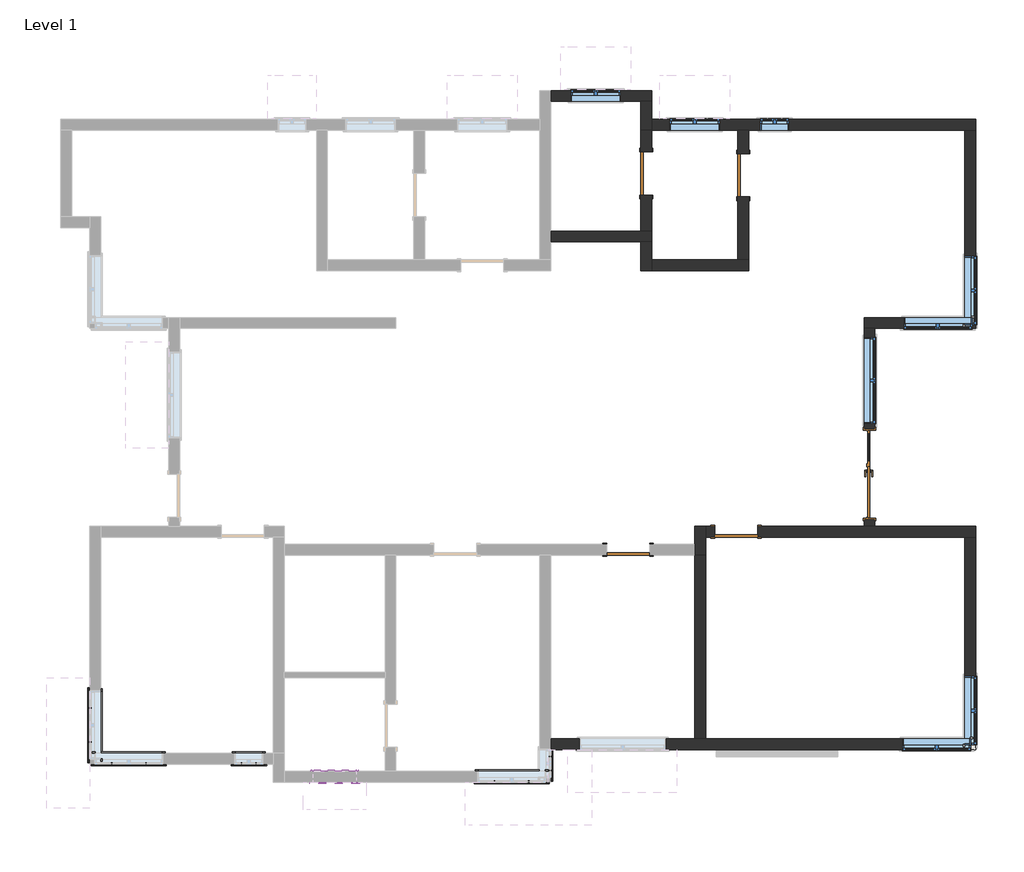
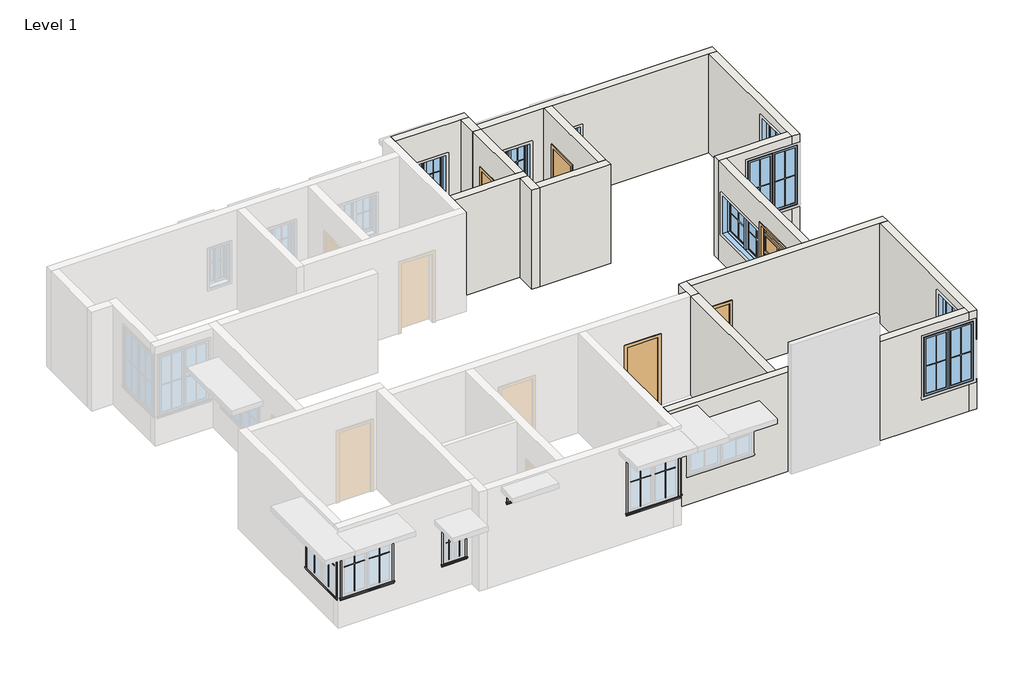
# One storey, part 2 of 3: 23 proxies, 16 walls, 8 windows, 5 doors.
"""IFC4 building model written with IfcOpenShell, lengths in millimetres."""

from ifc_helpers import new_model, si_unit, frame, origin, origin_with_axes, place, context, project, spatial, polyline, outline, extrude, faceted_brep, transform, mapped, element, save
from components import muntin_pattern_2x2_muntin_pattern_2x2_ddac5204, muntin_pattern_2x2_muntin_pattern_2x2_784a3213, muntin_pattern_2x2_muntin_pattern_2x2_1c5971db, muntin_pattern_2x2_muntin_pattern_2x2_604ffb00, muntin_pattern_2x2_muntin_pattern_2x2_bff912c5, muntin_pattern_2x2_muntin_pattern_2x2_c2194282, muntin_pattern_2x2_muntin_pattern_2x2_cdee2e69, muntin_pattern_2x2_muntin_pattern_2x2_c5f040ee, trim_window_exterior_flat_with_sill_35723329, trim_window_exterior_flat_with_sill_3de9c0e0, trim_window_exterior_flat_with_sill_e04b3088, trim_window_exterior_flat_with_sill_19508c7d, trim_window_interior_flat_picture_frame_e16bff95, trim_window_interior_flat_picture_frame_a780e5c2, trim_window_interior_flat_picture_frame_2a7685fe, main_entrance_door_11153_main_entrance_door_11153_94c2f9e1, door_0ca8825f, window_782a76c6, window_2032b2cd, window_9ac97e1a, window_bf2f09a8

model = new_model("IFC4")

# Units and contexts
model_context = context("Model", 3, world=origin())
ifc_project = project(units=[si_unit("LENGTHUNIT", "METRE", prefix="MILLI")], contexts=[model_context])

# Site, building, storey
site = spatial("IfcSite", under=ifc_project)
building = spatial("IfcBuilding", under=site)
storey = spatial("IfcBuildingStorey", under=building, Name="Level 1", Elevation=0.0)

# Proxies
placement = place(None, origin())
muntin_pattern_2x2_muntin_pattern_2x2_shape = muntin_pattern_2x2_muntin_pattern_2x2_ddac5204(model_context)
element("IfcBuildingElementProxy", 1, Name="Muntin Pattern_2x2 : Muntin Pattern_2x2", ObjectType="Muntin Pattern_2x2 : Muntin Pattern_2x2", at=placement, inside=storey, context=model_context, shape_type="MappedRepresentation", body=[
    mapped(muntin_pattern_2x2_muntin_pattern_2x2_shape, transform((-38557.3020004, 6033.4506148, 984.25), x_axis=(-1.0, 0.0, 0.0), y_axis=(0.0, -1.0, 0.0), z_axis=(0.0, 0.0, 1.0))),
])
muntin_pattern_2x2_muntin_pattern_2x2_2_shape = muntin_pattern_2x2_muntin_pattern_2x2_784a3213(model_context)
element("IfcBuildingElementProxy", 2, Name="Muntin Pattern_2x2 : Muntin Pattern_2x2", ObjectType="Muntin Pattern_2x2 : Muntin Pattern_2x2", at=placement, inside=storey, context=model_context, shape_type="MappedRepresentation", body=[
    mapped(muntin_pattern_2x2_muntin_pattern_2x2_2_shape, transform((-38858.9270004, 6033.4506148, 984.25), x_axis=(1.0, 0.0, 0.0), y_axis=(0.0, 1.0, 0.0), z_axis=(0.0, 0.0, 1.0))),
])
muntin_pattern_2x2_muntin_pattern_2x2_3_shape = muntin_pattern_2x2_muntin_pattern_2x2_1c5971db(model_context)
element("IfcBuildingElementProxy", 3, Name="Muntin Pattern_2x2 : Muntin Pattern_2x2", ObjectType="Muntin Pattern_2x2 : Muntin Pattern_2x2", at=placement, inside=storey, context=model_context, shape_type="MappedRepresentation", body=[
    mapped(muntin_pattern_2x2_muntin_pattern_2x2_3_shape, transform((-36665.0020004, 5652.3722085, 2546.35), x_axis=(-1.0, 0.0, 0.0), y_axis=(0.0, -1.0, 0.0), z_axis=(0.0, 0.0, 1.0))),
])
muntin_pattern_2x2_muntin_pattern_2x2_4_shape = muntin_pattern_2x2_muntin_pattern_2x2_604ffb00(model_context)
element("IfcBuildingElementProxy", 4, Name="Muntin Pattern_2x2 : Muntin Pattern_2x2", ObjectType="Muntin Pattern_2x2 : Muntin Pattern_2x2", at=placement, inside=storey, context=model_context, shape_type="MappedRepresentation", body=[
    mapped(muntin_pattern_2x2_muntin_pattern_2x2_4_shape, transform((-37119.0270004, 5652.3722085, 2546.35), x_axis=(1.0, 0.0, 0.0), y_axis=(0.0, 1.0, 0.0), z_axis=(0.0, 0.0, 1.0))),
])
muntin_pattern_2x2_muntin_pattern_2x2_5_shape = muntin_pattern_2x2_muntin_pattern_2x2_bff912c5(model_context)
element("IfcBuildingElementProxy", 5, Name="Muntin Pattern_2x2 : Muntin Pattern_2x2", ObjectType="Muntin Pattern_2x2 : Muntin Pattern_2x2", at=placement, inside=storey, context=model_context, shape_type="MappedRepresentation", body=[
    mapped(muntin_pattern_2x2_muntin_pattern_2x2_5_shape, transform((-32785.1520004, 5652.3722085, 984.25), x_axis=(-1.0, 0.0, 0.0), y_axis=(0.0, -1.0, 0.0), z_axis=(0.0, 0.0, 1.0))),
])
element("IfcBuildingElementProxy", 6, Name="Muntin Pattern_2x2 : Muntin Pattern_2x2", ObjectType="Muntin Pattern_2x2 : Muntin Pattern_2x2", at=placement, inside=storey, context=model_context, shape_type="MappedRepresentation", body=[
    mapped(muntin_pattern_2x2_muntin_pattern_2x2_5_shape, transform((-40887.7520004, 6033.4506148, 984.25), x_axis=(-1.0, 0.0, 0.0), y_axis=(0.0, -1.0, 0.0), z_axis=(0.0, 0.0, 1.0))),
])
element("IfcBuildingElementProxy", 7, Name="Muntin Pattern_2x2 : Muntin Pattern_2x2", ObjectType="Muntin Pattern_2x2 : Muntin Pattern_2x2", at=placement, inside=storey, context=model_context, shape_type="MappedRepresentation", body=[
    mapped(muntin_pattern_2x2_muntin_pattern_2x2_5_shape, transform((-42064.0895004, 6489.0631148, 984.25), x_axis=(0.0, 1.0, 0.0), y_axis=(-1.0, 0.0, 0.0), z_axis=(0.0, 0.0, 1.0))),
])
muntin_pattern_2x2_muntin_pattern_2x2_6_shape = muntin_pattern_2x2_muntin_pattern_2x2_c2194282(model_context)
element("IfcBuildingElementProxy", 8, Name="Muntin Pattern_2x2 : Muntin Pattern_2x2", ObjectType="Muntin Pattern_2x2 : Muntin Pattern_2x2", at=placement, inside=storey, context=model_context, shape_type="MappedRepresentation", body=[
    mapped(muntin_pattern_2x2_muntin_pattern_2x2_6_shape, transform((-33505.8770004, 5652.3722085, 984.25), x_axis=(1.0, 0.0, 0.0), y_axis=(0.0, 1.0, 0.0), z_axis=(0.0, 0.0, 1.0))),
])
element("IfcBuildingElementProxy", 9, Name="Muntin Pattern_2x2 : Muntin Pattern_2x2", ObjectType="Muntin Pattern_2x2 : Muntin Pattern_2x2", at=placement, inside=storey, context=model_context, shape_type="MappedRepresentation", body=[
    mapped(muntin_pattern_2x2_muntin_pattern_2x2_6_shape, transform((-41608.4770004, 6033.4506148, 984.25), x_axis=(1.0, 0.0, 0.0), y_axis=(0.0, 1.0, 0.0), z_axis=(0.0, 0.0, 1.0))),
])
element("IfcBuildingElementProxy", 10, Name="Muntin Pattern_2x2 : Muntin Pattern_2x2", ObjectType="Muntin Pattern_2x2 : Muntin Pattern_2x2", at=placement, inside=storey, context=model_context, shape_type="MappedRepresentation", body=[
    mapped(muntin_pattern_2x2_muntin_pattern_2x2_6_shape, transform((-42064.0895004, 7209.7881148, 984.25), x_axis=(0.0, -1.0, 0.0), y_axis=(1.0, 0.0, 0.0), z_axis=(0.0, 0.0, 1.0))),
])
muntin_pattern_2x2_muntin_pattern_2x2_7_shape = muntin_pattern_2x2_muntin_pattern_2x2_cdee2e69(model_context)
element("IfcBuildingElementProxy", 11, Name="Muntin Pattern_2x2 : Muntin Pattern_2x2", ObjectType="Muntin Pattern_2x2 : Muntin Pattern_2x2", at=placement, inside=storey, context=model_context, shape_type="MappedRepresentation", body=[
    mapped(muntin_pattern_2x2_muntin_pattern_2x2_7_shape, transform((-32329.5395004, 6187.3597085, 984.25), x_axis=(0.0, -1.0, 0.0), y_axis=(1.0, 0.0, 0.0), z_axis=(0.0, 0.0, 1.0))),
])
muntin_pattern_2x2_muntin_pattern_2x2_8_shape = muntin_pattern_2x2_muntin_pattern_2x2_c5f040ee(model_context)
element("IfcBuildingElementProxy", 12, Name="Muntin Pattern_2x2 : Muntin Pattern_2x2", ObjectType="Muntin Pattern_2x2 : Muntin Pattern_2x2", at=placement, inside=storey, context=model_context, shape_type="MappedRepresentation", body=[
    mapped(muntin_pattern_2x2_muntin_pattern_2x2_8_shape, transform((-32329.5395004, 5885.7347085, 984.25), x_axis=(0.0, 1.0, 0.0), y_axis=(-1.0, 0.0, 0.0), z_axis=(0.0, 0.0, 1.0))),
])
trim_window_exterior_flat_with_sill_shape = trim_window_exterior_flat_with_sill_35723329(model_context)
element("IfcBuildingElementProxy", 13, Name="Trim-Window-Exterior-Flat : with Sill", ObjectType="Trim-Window-Exterior-Flat : with Sill", at=placement, inside=storey, context=model_context, shape_type="MappedRepresentation", body=[
    mapped(trim_window_exterior_flat_with_sill_shape, transform((-38708.1145004, 6023.9256148, 2133.6), x_axis=(1.0, 0.0, 0.0), y_axis=(0.0, 0.0, 1.0), z_axis=(0.0, -1.0, 0.0))),
])
trim_window_exterior_flat_with_sill_2_shape = trim_window_exterior_flat_with_sill_3de9c0e0(model_context)
element("IfcBuildingElementProxy", 14, Name="Trim-Window-Exterior-Flat : with Sill", ObjectType="Trim-Window-Exterior-Flat : with Sill", at=placement, inside=storey, context=model_context, shape_type="MappedRepresentation", body=[
    mapped(trim_window_exterior_flat_with_sill_2_shape, transform((-36892.0145004, 5642.8472085, 2781.3), x_axis=(1.0, 0.0, 0.0), y_axis=(0.0, 0.0, 1.0), z_axis=(0.0, -1.0, 0.0))),
])
trim_window_exterior_flat_with_sill_3_shape = trim_window_exterior_flat_with_sill_e04b3088(model_context)
element("IfcBuildingElementProxy", 15, Name="Trim-Window-Exterior-Flat : with Sill", ObjectType="Trim-Window-Exterior-Flat : with Sill", at=placement, inside=storey, context=model_context, shape_type="MappedRepresentation", body=[
    mapped(trim_window_exterior_flat_with_sill_3_shape, transform((-33145.5145004, 5642.8472085, 2743.2), x_axis=(1.0, 0.0, 0.0), y_axis=(0.0, 0.0, 1.0), z_axis=(0.0, -1.0, 0.0))),
])
element("IfcBuildingElementProxy", 16, Name="Trim-Window-Exterior-Flat : with Sill", ObjectType="Trim-Window-Exterior-Flat : with Sill", at=placement, inside=storey, context=model_context, shape_type="MappedRepresentation", body=[
    mapped(trim_window_exterior_flat_with_sill_3_shape, transform((-41248.1145004, 6023.9256148, 2743.2), x_axis=(1.0, 0.0, 0.0), y_axis=(0.0, 0.0, 1.0), z_axis=(0.0, -1.0, 0.0))),
])
element("IfcBuildingElementProxy", 17, Name="Trim-Window-Exterior-Flat : with Sill", ObjectType="Trim-Window-Exterior-Flat : with Sill", at=placement, inside=storey, context=model_context, shape_type="MappedRepresentation", body=[
    mapped(trim_window_exterior_flat_with_sill_3_shape, transform((-42073.6145004, 6849.4256148, 2743.2), x_axis=(0.0, -1.0, 0.0), y_axis=(0.0, 0.0, 1.0), z_axis=(-1.0, 0.0, 0.0))),
])
trim_window_exterior_flat_with_sill_4_shape = trim_window_exterior_flat_with_sill_19508c7d(model_context)
element("IfcBuildingElementProxy", 18, Name="Trim-Window-Exterior-Flat : with Sill", ObjectType="Trim-Window-Exterior-Flat : with Sill", at=placement, inside=storey, context=model_context, shape_type="MappedRepresentation", body=[
    mapped(trim_window_exterior_flat_with_sill_4_shape, transform((-32320.0145004, 6036.5472085, 2743.2), x_axis=(0.0, 1.0, 0.0), y_axis=(0.0, 0.0, 1.0), z_axis=(1.0, 0.0, 0.0))),
])
trim_window_interior_flat_picture_frame_shape = trim_window_interior_flat_picture_frame_e16bff95(model_context)
element("IfcBuildingElementProxy", 19, Name="Trim-Window-Interior-Flat : Picture Frame", ObjectType="Trim-Window-Interior-Flat : Picture Frame", at=placement, inside=storey, context=model_context, shape_type="MappedRepresentation", body=[
    mapped(trim_window_interior_flat_picture_frame_shape, transform((-38708.1145004, 6252.5256148, 2133.6), x_axis=(-1.0, 0.0, 0.0), y_axis=(0.0, 0.0, 1.0), z_axis=(0.0, 1.0, 0.0))),
])
trim_window_interior_flat_picture_frame_2_shape = trim_window_interior_flat_picture_frame_a780e5c2(model_context)
element("IfcBuildingElementProxy", 20, Name="Trim-Window-Interior-Flat : Picture Frame", ObjectType="Trim-Window-Interior-Flat : Picture Frame", at=placement, inside=storey, context=model_context, shape_type="MappedRepresentation", body=[
    mapped(trim_window_interior_flat_picture_frame_2_shape, transform((-36892.0145004, 5871.4472085, 2781.3), x_axis=(-1.0, 0.0, 0.0), y_axis=(0.0, 0.0, 1.0), z_axis=(0.0, 1.0, 0.0))),
])
trim_window_interior_flat_picture_frame_3_shape = trim_window_interior_flat_picture_frame_2a7685fe(model_context)
element("IfcBuildingElementProxy", 21, Name="Trim-Window-Interior-Flat : Picture Frame", ObjectType="Trim-Window-Interior-Flat : Picture Frame", at=placement, inside=storey, context=model_context, shape_type="MappedRepresentation", body=[
    mapped(trim_window_interior_flat_picture_frame_3_shape, transform((-33145.5145004, 5871.4472085, 2743.2), x_axis=(-1.0, 0.0, 0.0), y_axis=(0.0, 0.0, 1.0), z_axis=(0.0, 1.0, 0.0))),
])
element("IfcBuildingElementProxy", 22, Name="Trim-Window-Interior-Flat : Picture Frame", ObjectType="Trim-Window-Interior-Flat : Picture Frame", at=placement, inside=storey, context=model_context, shape_type="MappedRepresentation", body=[
    mapped(trim_window_interior_flat_picture_frame_3_shape, transform((-41248.1145004, 6252.5256148, 2743.2), x_axis=(-1.0, 0.0, 0.0), y_axis=(0.0, 0.0, 1.0), z_axis=(0.0, 1.0, 0.0))),
])
element("IfcBuildingElementProxy", 23, Name="Trim-Window-Interior-Flat : Picture Frame", ObjectType="Trim-Window-Interior-Flat : Picture Frame", at=placement, inside=storey, context=model_context, shape_type="MappedRepresentation", body=[
    mapped(trim_window_interior_flat_picture_frame_3_shape, transform((-41845.0145004, 6849.4256148, 2743.2), x_axis=(0.0, 1.0, 0.0), y_axis=(0.0, 0.0, 1.0), z_axis=(1.0, 0.0, 0.0))),
])

# Doors
main_entrance_door_11153_main_entrance_door_11153_shape = main_entrance_door_11153_main_entrance_door_11153_94c2f9e1(model_context)
element("IfcDoor", 24, ObjectType="Main_entrance_door_11153 : Main_entrance_door_11153", at=placement, inside=storey, context=model_context, shape_type="MappedRepresentation", body=[
    mapped(main_entrance_door_11153_main_entrance_door_11153_shape, transform((-25576.3145004, 12158.0256148, 0.0), x_axis=(0.0, 1.0, 0.0), y_axis=(-1.0, 0.0, 0.0), z_axis=(0.0, 0.0, 1.0))),
])
door_shape = door_0ca8825f(model_context)
element("IfcDoor", 25, ObjectType="Single-Flush : 36\" x 84\"", at=placement, inside=storey, context=model_context, shape_type="MappedRepresentation", body=[
    mapped(door_shape, transform((-28395.7145004, 10938.8256148, 0.0), x_axis=(-1.0, 0.0, 0.0), y_axis=(0.0, -1.0, 0.0), z_axis=(0.0, 0.0, 1.0))),
])
element("IfcDoor", 26, ObjectType="Single-Flush : 36\" x 84\"", at=placement, inside=storey, context=model_context, shape_type="MappedRepresentation", body=[
    mapped(door_shape, transform((-28243.3145004, 18482.6256148, 0.0), x_axis=(0.0, 1.0, 0.0), y_axis=(-1.0, 0.0, 0.0), z_axis=(0.0, 0.0, 1.0))),
])
element("IfcDoor", 27, ObjectType="Single-Flush : 36\" x 84\"", at=placement, inside=storey, context=model_context, shape_type="MappedRepresentation", body=[
    mapped(door_shape, transform((-30300.7145004, 18520.7256148, 0.0), x_axis=(0.0, 1.0, 0.0), y_axis=(-1.0, 0.0, 0.0), z_axis=(0.0, 0.0, 1.0))),
])
element("IfcDoor", 28, ObjectType="Single-Flush : 36\" x 84\"", at=placement, inside=storey, context=model_context, shape_type="MappedRepresentation", body=[
    mapped(door_shape, transform((-30681.7145004, 10557.8256148, 0.0), x_axis=(-1.0, 0.0, 0.0), y_axis=(0.0, -1.0, 0.0), z_axis=(0.0, 0.0, 1.0))),
])

# Walls
element("IfcWall", 29, ObjectType="wall 9\"", at=placement, inside=storey, context=model_context, shape_type="Brep", body=[
    faceted_brep([(-32320.0145004, 20044.7256148, 0.0), (-30415.0145004, 20044.7256148, 0.0), (-30186.4145004, 20044.7256148, 0.0), (-30186.4145004, 20044.7256148, 3048.0), (-30415.0145004, 20044.7256148, 3048.0), (-32320.0145004, 20044.7256148, 3048.0), (-30834.1145004, 20044.7256148, 2133.6), (-30834.1145004, 20044.7256148, 914.4), (-31900.9145004, 20044.7256148, 914.4), (-31900.9145004, 20044.7256148, 2133.6), (-32320.0145004, 20273.3256148, 0.0), (-32320.0145004, 20273.3256148, 3048.0), (-30186.4145004, 20273.3256148, 3048.0), (-30186.4145004, 20273.3256148, 0.0), (-30834.1145004, 20273.3256148, 2133.6), (-31900.9145004, 20273.3256148, 2133.6), (-31900.9145004, 20273.3256148, 914.4), (-30834.1145004, 20273.3256148, 914.4)], [[[0, 1, 2, 3, 4, 5], [6, 7, 8, 9]], [[10, 11, 12, 13], [14, 15, 16, 17]], [[2, 1, 0, 10, 13]], [[5, 4, 3, 12, 11]], [[0, 5, 11, 10]], [[3, 2, 13, 12]], [[7, 6, 14, 17]], [[8, 7, 17, 16]], [[9, 8, 16, 15]], [[6, 9, 15, 14]]]),
])
element("IfcWall", 30, ObjectType="wall 9\"", at=placement, inside=storey, context=model_context, shape_type="Brep", body=[
    faceted_brep([(-30415.0145004, 20044.7256148, 0.0), (-30415.0145004, 19435.1256148, 0.0), (-30415.0145004, 19435.1256148, 3048.0), (-30415.0145004, 20044.7256148, 3048.0), (-30186.4145004, 20044.7256148, 0.0), (-30186.4145004, 20044.7256148, 3048.0), (-30186.4145004, 19663.7256148, 3048.0), (-30186.4145004, 19435.1256148, 3048.0), (-30186.4145004, 19435.1256148, 0.0), (-30186.4145004, 19663.7256148, 0.0)], [[[0, 1, 2, 3]], [[4, 5, 6, 7, 8, 9]], [[1, 0, 4, 9, 8]], [[3, 2, 7, 6, 5]], [[0, 3, 5, 4]], [[2, 1, 8, 7]]]),
])
element("IfcWall", 31, ObjectType="wall 9\"", at=placement, inside=storey, context=model_context, shape_type="Brep", body=[
    faceted_brep([(-30186.4145004, 19435.1256148, 0.0), (-28357.6145004, 19435.1256148, 0.0), (-28129.0145004, 19435.1256148, 0.0), (-23557.0145004, 19435.1256148, 0.0), (-23328.4145004, 19435.1256148, 0.0), (-23328.4145004, 19435.1256148, 3048.0), (-23557.0145004, 19435.1256148, 3048.0), (-28129.0145004, 19435.1256148, 3048.0), (-28357.6145004, 19435.1256148, 3048.0), (-30186.4145004, 19435.1256148, 3048.0), (-27278.1145004, 19435.1256148, 2133.6), (-27278.1145004, 19435.1256148, 914.4), (-27887.7145004, 19435.1256148, 914.4), (-27887.7145004, 19435.1256148, 2133.6), (-28738.6145004, 19435.1256148, 2133.6), (-28738.6145004, 19435.1256148, 914.4), (-29805.4145004, 19435.1256148, 914.4), (-29805.4145004, 19435.1256148, 2133.6), (-30186.4145004, 19663.7256148, 0.0), (-30186.4145004, 19663.7256148, 3048.0), (-23328.4145004, 19663.7256148, 3048.0), (-23328.4145004, 19663.7256148, 0.0), (-27278.1145004, 19663.7256148, 2133.6), (-27887.7145004, 19663.7256148, 2133.6), (-27887.7145004, 19663.7256148, 914.4), (-27278.1145004, 19663.7256148, 914.4), (-28738.6145004, 19663.7256148, 2133.6), (-29805.4145004, 19663.7256148, 2133.6), (-29805.4145004, 19663.7256148, 914.4), (-28738.6145004, 19663.7256148, 914.4)], [[[0, 1, 2, 3, 4, 5, 6, 7, 8, 9], [10, 11, 12, 13], [14, 15, 16, 17]], [[18, 19, 20, 21], [22, 23, 24, 25], [26, 27, 28, 29]], [[1, 0, 18, 21, 4, 3, 2]], [[6, 5, 20, 19, 9, 8, 7]], [[0, 9, 19, 18]], [[5, 4, 21, 20]], [[15, 14, 26, 29]], [[16, 15, 29, 28]], [[17, 16, 28, 27]], [[14, 17, 27, 26]], [[11, 10, 22, 25]], [[12, 11, 25, 24]], [[13, 12, 24, 23]], [[10, 13, 23, 22]]]),
])
element("IfcWall", 32, ObjectType="wall 9\"", at=placement, inside=storey, context=model_context, shape_type="Brep", body=[
    faceted_brep([(-23557.0145004, 19435.1256148, 0.0), (-23557.0145004, 15472.7256148, 0.0), (-23557.0145004, 15244.1256148, 0.0), (-23557.0145004, 15244.1256148, 914.4), (-23557.0145004, 15472.7256148, 914.4), (-23557.0145004, 16768.1256148, 914.4), (-23557.0145004, 16768.1256148, 2743.2), (-23557.0145004, 15472.7256148, 2743.2), (-23557.0145004, 15244.1256148, 2743.2), (-23557.0145004, 15244.1256148, 3048.0), (-23557.0145004, 15472.7256148, 3048.0), (-23557.0145004, 19435.1256148, 3048.0), (-23328.4145004, 15244.1256148, 0.0), (-23328.4145004, 19435.1256148, 0.0), (-23328.4145004, 19435.1256148, 3048.0), (-23328.4145004, 15244.1256148, 3048.0), (-23328.4145004, 15320.3256148, 914.4), (-23328.4145004, 15320.3256148, 2743.2), (-23328.4145004, 16768.1256148, 2743.2), (-23328.4145004, 16768.1256148, 914.4), (-23404.6145004, 15244.1256148, 2743.2), (-23404.6145004, 15244.1256148, 914.4), (-23404.6145004, 15320.3256148, 914.4), (-23404.6145004, 15320.3256148, 2743.2)], [[[0, 1, 2, 3, 4, 5, 6, 7, 8, 9, 10, 11]], [[12, 13, 14, 15], [16, 17, 18, 19]], [[2, 1, 0, 13, 12]], [[11, 10, 9, 15, 14]], [[0, 11, 14, 13]], [[2, 12, 15, 9, 8, 20, 21, 3]], [[3, 21, 22, 16, 19, 5, 4]], [[21, 20, 23, 22]], [[20, 8, 7, 6, 18, 17, 23]], [[23, 17, 16, 22]], [[5, 19, 18, 6]]]),
])
element("IfcWall", 33, ObjectType="wall 9\"", at=placement, inside=storey, context=model_context, shape_type="Brep", body=[
    faceted_brep([(-23557.0145004, 15472.7256148, 0.0), (-25690.6145004, 15472.7256148, 0.0), (-25690.6145004, 15472.7256148, 3048.0), (-23557.0145004, 15472.7256148, 3048.0), (-23557.0145004, 15472.7256148, 2743.2), (-24852.4145004, 15472.7256148, 2743.2), (-24852.4145004, 15472.7256148, 914.4), (-23557.0145004, 15472.7256148, 914.4), (-25690.6145004, 15244.1256148, 0.0), (-25462.0145004, 15244.1256148, 0.0), (-23557.0145004, 15244.1256148, 0.0), (-23557.0145004, 15244.1256148, 914.4), (-24852.4145004, 15244.1256148, 914.4), (-24852.4145004, 15244.1256148, 2743.2), (-23557.0145004, 15244.1256148, 2743.2), (-23557.0145004, 15244.1256148, 3048.0), (-25462.0145004, 15244.1256148, 3048.0), (-25690.6145004, 15244.1256148, 3048.0)], [[[0, 1, 2, 3, 4, 5, 6, 7]], [[8, 9, 10, 11, 12, 13, 14, 15, 16, 17]], [[1, 0, 10, 9, 8]], [[3, 2, 17, 16, 15]], [[0, 7, 11, 10]], [[2, 1, 8, 17]], [[6, 5, 13, 12]], [[7, 6, 12, 11]], [[5, 4, 14, 13]], [[4, 3, 15, 14]]]),
])
element("IfcWall", 34, ObjectType="wall 9\"", at=placement, inside=storey, context=model_context, shape_type="SweptSolid", body=[
    extrude(outline(polyline([(11053.1256148, 3048.0), (15244.1256148, 3048.0), (15244.1256148, 0.0), (13108.0256148, 0.0), (13108.0256148, 2400.0), (11208.0256148, 2400.0), (11208.0256148, 0.0), (11053.1256148, 0.0), (11053.1256148, 3048.0)]), holes=[polyline([(13224.8256148, 2133.6), (13224.8256148, 914.4), (15053.6256148, 914.4), (15053.6256148, 2133.6), (13224.8256148, 2133.6)])]), frame((-25690.6145004, 0.0, 0.0), z_axis=(1.0, 0.0, 0.0), x_axis=(0.0, 1.0, 0.0)), (0.0, 0.0, 1.0), 228.6),
])
element("IfcWall", 35, ObjectType="wall 9\"", at=placement, inside=storey, context=model_context, shape_type="Brep", body=[
    faceted_brep([(-29043.4145004, 10824.5256148, 0.0), (-28852.9145004, 10824.5256148, 0.0), (-28852.9145004, 10824.5256148, 2133.6), (-27938.5145004, 10824.5256148, 2133.6), (-27938.5145004, 10824.5256148, 0.0), (-23557.0145004, 10824.5256148, 0.0), (-23328.4145004, 10824.5256148, 0.0), (-23328.4145004, 10824.5256148, 3048.0), (-23557.0145004, 10824.5256148, 3048.0), (-29043.4145004, 10824.5256148, 3048.0), (-28852.9145004, 11053.1256148, 2133.6), (-28852.9145004, 11053.1256148, 0.0), (-29043.4145004, 11053.1256148, 0.0), (-29043.4145004, 11053.1256148, 3048.0), (-25690.6145004, 11053.1256148, 3048.0), (-25462.0145004, 11053.1256148, 3048.0), (-23328.4145004, 11053.1256148, 3048.0), (-23328.4145004, 11053.1256148, 0.0), (-25462.0145004, 11053.1256148, 0.0), (-25690.6145004, 11053.1256148, 0.0), (-27938.5145004, 11053.1256148, 0.0), (-27938.5145004, 11053.1256148, 2133.6)], [[[0, 1, 2, 3, 4, 5, 6, 7, 8, 9]], [[10, 11, 12, 13, 14, 15, 16, 17, 18, 19, 20, 21]], [[12, 11, 1, 0]], [[20, 19, 18, 17, 6, 5, 4]], [[9, 8, 7, 16, 15, 14, 13]], [[7, 6, 17, 16]], [[0, 9, 13, 12]], [[2, 1, 11, 10]], [[3, 2, 10, 21]], [[4, 3, 21, 20]]]),
])
element("IfcWall", 36, ObjectType="wall 9\"", at=placement, inside=storey, context=model_context, shape_type="Brep", body=[
    faceted_brep([(-23557.0145004, 10824.5256148, 0.0), (-23557.0145004, 6557.3256148, 0.0), (-23557.0145004, 6328.7256148, 0.0), (-23557.0145004, 6328.7256148, 914.4), (-23557.0145004, 6557.3256148, 914.4), (-23557.0145004, 7878.1256148, 914.4), (-23557.0145004, 7878.1256148, 2743.2), (-23557.0145004, 6557.3256148, 2743.2), (-23557.0145004, 6328.7256148, 2743.2), (-23557.0145004, 6328.7256148, 3048.0), (-23557.0145004, 6557.3256148, 3048.0), (-23557.0145004, 10824.5256148, 3048.0), (-23328.4145004, 6328.7256148, 0.0), (-23328.4145004, 10824.5256148, 0.0), (-23328.4145004, 10824.5256148, 3048.0), (-23328.4145004, 6328.7256148, 3048.0), (-23328.4145004, 6328.7256148, 2133.6), (-23328.4145004, 6430.3256148, 2133.6), (-23328.4145004, 6430.3256148, 2743.2), (-23328.4145004, 7878.1256148, 2743.2), (-23328.4145004, 7878.1256148, 914.4), (-23328.4145004, 6328.7256148, 914.4), (-23430.0145004, 6328.7256148, 2133.6), (-23430.0145004, 6430.3256148, 2133.6), (-23430.0145004, 6328.7256148, 2743.2), (-23430.0145004, 6430.3256148, 2743.2)], [[[0, 1, 2, 3, 4, 5, 6, 7, 8, 9, 10, 11]], [[12, 13, 14, 15, 16, 17, 18, 19, 20, 21]], [[2, 1, 0, 13, 12]], [[11, 10, 9, 15, 14]], [[0, 11, 14, 13]], [[16, 22, 23, 17]], [[20, 5, 4, 3, 21]], [[2, 12, 21, 3]], [[15, 9, 8, 24, 22, 16]], [[22, 24, 25, 23]], [[24, 8, 7, 6, 19, 18, 25]], [[25, 18, 17, 23]], [[5, 20, 19, 6]]]),
])
element("IfcWall", 37, ObjectType="wall 9\"", at=placement, inside=storey, context=model_context, shape_type="Brep", body=[
    faceted_brep([(-23557.0145004, 6557.3256148, 0.0), (-29043.4145004, 6557.3256148, 0.0), (-29272.0145004, 6557.3256148, 0.0), (-32320.0145004, 6557.3256148, 0.0), (-32320.0145004, 6557.3256148, 3048.0), (-29272.0145004, 6557.3256148, 3048.0), (-29043.4145004, 6557.3256148, 3048.0), (-23557.0145004, 6557.3256148, 3048.0), (-23557.0145004, 6557.3256148, 2743.2), (-24877.8145004, 6557.3256148, 2743.2), (-24877.8145004, 6557.3256148, 914.4), (-23557.0145004, 6557.3256148, 914.4), (-31710.4145004, 6557.3256148, 2133.6), (-31710.4145004, 6557.3256148, 914.4), (-29881.6145004, 6557.3256148, 914.4), (-29881.6145004, 6557.3256148, 2133.6), (-32320.0145004, 6328.7256148, 0.0), (-23557.0145004, 6328.7256148, 0.0), (-23557.0145004, 6328.7256148, 914.4), (-24877.8145004, 6328.7256148, 914.4), (-24877.8145004, 6328.7256148, 2743.2), (-23557.0145004, 6328.7256148, 2743.2), (-23557.0145004, 6328.7256148, 3048.0), (-32320.0145004, 6328.7256148, 3048.0), (-31710.4145004, 6328.7256148, 2133.6), (-29881.6145004, 6328.7256148, 2133.6), (-29881.6145004, 6328.7256148, 914.4), (-31710.4145004, 6328.7256148, 914.4)], [[[0, 1, 2, 3, 4, 5, 6, 7, 8, 9, 10, 11], [12, 13, 14, 15]], [[16, 17, 18, 19, 20, 21, 22, 23], [24, 25, 26, 27]], [[1, 0, 17, 16, 3, 2]], [[5, 4, 23, 22, 7, 6]], [[4, 3, 16, 23]], [[13, 12, 24, 27]], [[14, 13, 27, 26]], [[15, 14, 26, 25]], [[12, 15, 25, 24]], [[11, 10, 19, 18]], [[8, 7, 22, 21]], [[0, 11, 18, 17]], [[10, 9, 20, 19]], [[9, 8, 21, 20]]]),
])
element("IfcWall", 38, ObjectType="wall 9\"", at=placement, inside=storey, context=model_context, shape_type="Brep", body=[
    faceted_brep([(-32320.0145004, 17072.9256148, 0.0), (-30415.0145004, 17072.9256148, 0.0), (-30186.4145004, 17072.9256148, 0.0), (-30186.4145004, 17072.9256148, 3048.0), (-30415.0145004, 17072.9256148, 3048.0), (-32320.0145004, 17072.9256148, 3048.0), (-32320.0145004, 17301.5256148, 0.0), (-32320.0145004, 17301.5256148, 3048.0), (-30415.0145004, 17301.5256148, 3048.0), (-30186.4145004, 17301.5256148, 3048.0), (-30186.4145004, 17301.5256148, 0.0), (-30415.0145004, 17301.5256148, 0.0)], [[[0, 1, 2, 3, 4, 5]], [[6, 7, 8, 9, 10, 11]], [[2, 1, 0, 6, 11, 10]], [[5, 4, 3, 9, 8, 7]], [[0, 5, 7, 6]], [[3, 2, 10, 9]]]),
])
element("IfcWall", 39, ObjectType="wall 9\"", at=placement, inside=storey, context=model_context, shape_type="Brep", body=[
    faceted_brep([(-30415.0145004, 17072.9256148, 0.0), (-30415.0145004, 16463.3256148, 0.0), (-30415.0145004, 16463.3256148, 3048.0), (-30415.0145004, 17072.9256148, 3048.0), (-30186.4145004, 17072.9256148, 0.0), (-30186.4145004, 17072.9256148, 3048.0), (-30186.4145004, 16691.9256148, 3048.0), (-30186.4145004, 16463.3256148, 3048.0), (-30186.4145004, 16463.3256148, 0.0), (-30186.4145004, 16691.9256148, 0.0)], [[[0, 1, 2, 3]], [[4, 5, 6, 7, 8, 9]], [[1, 0, 4, 9, 8]], [[3, 2, 7, 6, 5]], [[0, 3, 5, 4]], [[2, 1, 8, 7]]]),
])
element("IfcWall", 40, ObjectType="wall 9\"", at=placement, inside=storey, context=model_context, shape_type="Brep", body=[
    faceted_brep([(-30186.4145004, 16463.3256148, 0.0), (-28129.0145004, 16463.3256148, 0.0), (-28129.0145004, 16463.3256148, 3048.0), (-30186.4145004, 16463.3256148, 3048.0), (-30186.4145004, 16691.9256148, 0.0), (-30186.4145004, 16691.9256148, 3048.0), (-28357.6145004, 16691.9256148, 3048.0), (-28129.0145004, 16691.9256148, 3048.0), (-28129.0145004, 16691.9256148, 0.0), (-28357.6145004, 16691.9256148, 0.0)], [[[0, 1, 2, 3]], [[4, 5, 6, 7, 8, 9]], [[1, 0, 4, 9, 8]], [[3, 2, 7, 6, 5]], [[0, 3, 5, 4]], [[2, 1, 8, 7]]]),
])
element("IfcWall", 41, ObjectType="wall 9\"", at=placement, inside=storey, context=model_context, shape_type="SweptSolid", body=[
    extrude(outline(polyline([(19435.1256148, 0.0), (18939.8256148, 0.0), (18939.8256148, 2133.6), (18025.4256148, 2133.6), (18025.4256148, 0.0), (16691.9256148, 0.0), (16691.9256148, 3048.0), (19435.1256148, 3048.0), (19435.1256148, 0.0)])), frame((-28357.6145004, 0.0, 0.0), z_axis=(1.0, 0.0, 0.0), x_axis=(0.0, 1.0, 0.0)), (0.0, 0.0, 1.0), 228.6),
])
element("IfcWall", 42, ObjectType="wall 9\"", at=placement, inside=storey, context=model_context, shape_type="SweptSolid", body=[
    extrude(outline(polyline([(19435.1256148, 0.0), (18977.9256148, 0.0), (18977.9256148, 2133.6), (18063.5256148, 2133.6), (18063.5256148, 0.0), (17301.5256148, 0.0), (17301.5256148, 3048.0), (19435.1256148, 3048.0), (19435.1256148, 0.0)])), frame((-30415.0145004, 0.0, 0.0), z_axis=(1.0, 0.0, 0.0), x_axis=(0.0, 1.0, 0.0)), (0.0, 0.0, 1.0), 228.6),
])
element("IfcWall", 43, ObjectType="wall 9\"", at=placement, inside=storey, context=model_context, shape_type="Brep", body=[
    faceted_brep([(-29043.4145004, 10443.5256148, 0.0), (-29043.4145004, 10824.5256148, 0.0), (-29043.4145004, 11053.1256148, 0.0), (-29043.4145004, 11053.1256148, 3048.0), (-29043.4145004, 10824.5256148, 3048.0), (-29043.4145004, 10443.5256148, 3048.0), (-29272.0145004, 10443.5256148, 0.0), (-29272.0145004, 10443.5256148, 3048.0), (-29272.0145004, 10672.1256148, 3048.0), (-29272.0145004, 11053.1256148, 3048.0), (-29272.0145004, 11053.1256148, 0.0), (-29272.0145004, 10672.1256148, 0.0)], [[[0, 1, 2, 3, 4, 5]], [[6, 7, 8, 9, 10, 11]], [[2, 1, 0, 6, 11, 10]], [[5, 4, 3, 9, 8, 7]], [[0, 5, 7, 6]], [[3, 2, 10, 9]]]),
])
element("IfcWall", 44, ObjectType="wall 9\"", at=placement, inside=storey, context=model_context, shape_type="SweptSolid", body=[
    extrude(outline(polyline([(-29272.0145004, 6557.3256148), (-29272.0145004, 10443.5256148), (-29043.4145004, 10443.5256148), (-29043.4145004, 6557.3256148), (-29272.0145004, 6557.3256148)])), origin_with_axes(), (0.0, 0.0, 1.0), 3048.0),
])

# Windows
window_shape = window_782a76c6(model_context)
element("IfcWindow", 45, ObjectType="Window-Casement-Double : 24\"X48\"", at=placement, inside=storey, context=model_context, shape_type="MappedRepresentation", body=[
    mapped(window_shape, transform((-27582.9145004, 19549.4256148, 0.0), x_axis=(1.0, 0.0, 0.0), y_axis=(0.0, 1.0, 0.0), z_axis=(0.0, 0.0, 1.0))),
])
window_2_shape = window_2032b2cd(model_context)
element("IfcWindow", 46, ObjectType="Window-Casement-Double : 42\"X48\"", at=placement, inside=storey, context=model_context, shape_type="MappedRepresentation", body=[
    mapped(window_2_shape, transform((-31367.5145004, 20159.0256148, 0.0), x_axis=(1.0, 0.0, 0.0), y_axis=(0.0, 1.0, 0.0), z_axis=(0.0, 0.0, 1.0))),
])
element("IfcWindow", 47, ObjectType="Window-Casement-Double : 42\"X48\"", at=placement, inside=storey, context=model_context, shape_type="MappedRepresentation", body=[
    mapped(window_2_shape, transform((-29272.0145004, 19549.4256148, 0.0), x_axis=(1.0, 0.0, 0.0), y_axis=(0.0, 1.0, 0.0), z_axis=(0.0, 0.0, 1.0))),
])
window_3_shape = window_9ac97e1a(model_context)
element("IfcWindow", 48, ObjectType="Window-Casement-Double : 57\" x 72\"", at=placement, inside=storey, context=model_context, shape_type="MappedRepresentation", body=[
    mapped(window_3_shape, transform((-24153.9145004, 6443.0256148, 0.0), x_axis=(-1.0, 0.0, 0.0), y_axis=(0.0, -1.0, 0.0), z_axis=(0.0, 0.0, 1.0))),
])
element("IfcWindow", 49, ObjectType="Window-Casement-Double : 57\" x 72\"", at=placement, inside=storey, context=model_context, shape_type="MappedRepresentation", body=[
    mapped(window_3_shape, transform((-23442.7145004, 7154.2256148, 0.0), x_axis=(0.0, -1.0, 0.0), y_axis=(1.0, 0.0, 0.0), z_axis=(0.0, 0.0, 1.0))),
])
element("IfcWindow", 50, ObjectType="Window-Casement-Double : 57\" x 72\"", at=placement, inside=storey, context=model_context, shape_type="MappedRepresentation", body=[
    mapped(window_3_shape, transform((-24128.5145004, 15358.4256148, 0.0), x_axis=(-1.0, 0.0, 0.0), y_axis=(0.0, -1.0, 0.0), z_axis=(0.0, 0.0, 1.0))),
])
element("IfcWindow", 51, ObjectType="Window-Casement-Double : 57\" x 72\"", at=placement, inside=storey, context=model_context, shape_type="MappedRepresentation", body=[
    mapped(window_3_shape, transform((-23442.7145004, 16044.2256148, 0.0), x_axis=(0.0, -1.0, 0.0), y_axis=(1.0, 0.0, 0.0), z_axis=(0.0, 0.0, 1.0))),
])
window_4_shape = window_bf2f09a8(model_context)
element("IfcWindow", 52, ObjectType="Window-Casement-Double : 72\"X48\" 2", at=placement, inside=storey, context=model_context, shape_type="MappedRepresentation", body=[
    mapped(window_4_shape, transform((-25576.3145004, 14139.2256148, 0.0), x_axis=(0.0, -1.0, 0.0), y_axis=(1.0, 0.0, 0.0), z_axis=(0.0, 0.0, 1.0))),
])

save(model, "model.ifc")

# Revit data of these elements
# Type "Muntin Pattern_2x2 : Muntin Pattern_2x2"
#   Width [instance default] = 4' - 0"
#   Thickness = 0' - 0 1/2"
#   Height [instance default] = 4' - 0"
#   Distance = 0' - 0 3/4"
#   Interior Material [instance default] = none
#   Exterior Material [instance default] = none
#   Default Elevation = 0
# Type "Trim-Window-Exterior-Flat : with Sill"
#   Trim Width = 0' - 2 1/4"
#   Trim Thickness_Picture Frame = 0' - 1 1/4"
#   Trim Thickness_with Sill = 0' - 0 3/4"
#   Sill Thickness = 0' - 1 1/4"
#   Opening Width [instance default] = 2' - 0"
#   Opening Height [instance default] = 3' - 0"
#   Default Elevation = 4' - 0"
#   Sill = yes
#   Picture Frame = no
#   Trim Material [instance default] = none
# Type "Trim-Window-Interior-Flat : Picture Frame"
#   Trim Thickness_Picture Frame = 0' - 1 1/4"
#   Trim Width = 0' - 2 1/4"
#   Trim Thickness_with Sill = 0' - 0 3/4"
#   Sill Thickness = 0' - 1 1/4"
#   Opening Width [instance default] = 2' - 0"
#   Opening Height [instance default] = 3' - 0"
#   Default Elevation = 4' - 0"
#   Sill = no
#   Picture Frame = yes
#   Trim Material [instance default] = none
# Type "Main_entrance_door_11153 : Main_entrance_door_11153"
#   Type Mark = "22"
#   Height = 7' - 10.48819"
#   Width = 6' - 2.80315"
#   Door Width = 3' - 7.30709"
#   Function = (empty or 0)
#   Wall Closure = (empty or 0)
# Type "Single-Flush : 36\" x 84\""
#   Type Mark = "1"
#   Construction Type Id = "MDOOR"
#   Assembly Code = "C1020"
#   Analytic Construction = "Metal"
#   Thickness = 0' - 2"
#   Heat Transfer Coefficient (U) = 0.651978 BTU/(h·ft²·°F)
#   Height = 7' - 0"
#   Trim Projection Ext = 0' - 1"
#   Trim Projection Int = 0' - 1"
#   Trim Width = 0' - 3"
#   Width = 3' - 0"
#   Define Thermal Properties by = 1
#   Define Thermal Properties by = 1
#   Door Material = Door - Panel
#   Frame Material = Door - Frame
#   Visual Light Transmittance = 0
#   Solar Heat Gain Coefficient = 0
#   Function = (empty or 0)
#   Wall Closure = (empty or 0)
# Type "wall 9\""
#   Assembly Code = "B2010"
#   Layers, outside or top first: 0' - 9" no material (function 1)
# Type "Window-Casement-Double : 24\"X48\""
#   Type Mark = "22"
#   Fire Rating = "0.5h"
#   Assembly Code = "B2020100"
#   Analytic Construction = "Double glazing - domestic"
#   Frame Extension [instance default] = 0' - 0 1/4"
#   Window Inset [instance default] = 0' - 0"
#   Wall Thickness [instance default] = 0' - 6"
#   Interior Wall Closure [instance default] = 0' - 2 1/4"
#   Half Width = 1' - 0"
#   Visual Light Transmittance = 0.81
#   Thermal Resistance (R) = 1.8146 (h·ft²·°F)/BTU
#   Solar Heat Gain Coefficient = 0.76
#   Rough Width = 2' - 0 1/2"
#   Rough Height = 4' - 0 1/2"
#   Height = 4' - 0"
#   Heat Transfer Coefficient (U) = 0.5511 BTU/(h·ft²·°F)
#   Exterior Wall Closure [instance default] = 0' - 1 1/4"
#   Extension Jamb [instance default] = 0' - 2 1/4"
#   Default Sill Height = 3' - 0"
#   Width = 2' - 0"
#   Muntin Visibility = yes
#   Interior Trim Visibility [instance default] = yes
#   Exterior Trim Visibility [instance default] = yes
#   Extension Jamb Visibility [instance default] = yes
#   Interior Trim Material = Wood - Stained
#   Muntin Pattern = Muntin Pattern_2x2 : Muntin Pattern_2x2
#   Interior Trim = Trim-Window-Interior-Flat : Picture Frame
#   Interior Frame Material = Wood - Stained
#   Glass Panel Material = Glass
#   Exterior Trim Material = Clad - White
#   Exterior Trim = Trim-Window-Exterior-Flat : with Sill
#   Exterior Frame Material = Clad - White
#   Wall Closure = (empty or 0)
# Type "Window-Casement-Double : 42\"X48\""
#   Type Mark = "27"
#   Fire Rating = "0.5h"
#   Assembly Code = "B2020100"
#   Analytic Construction = "Double glazing - domestic"
#   Frame Extension [instance default] = 0' - 0 1/4"
#   Window Inset [instance default] = 0' - 0"
#   Wall Thickness [instance default] = 0' - 6"
#   Interior Wall Closure [instance default] = 0' - 2 1/4"
#   Half Width = 1' - 9"
#   Visual Light Transmittance = 0.81
#   Thermal Resistance (R) = 1.8146 (h·ft²·°F)/BTU
#   Solar Heat Gain Coefficient = 0.76
#   Rough Width = 3' - 6 1/2"
#   Rough Height = 4' - 0 1/2"
#   Height = 4' - 0"
#   Heat Transfer Coefficient (U) = 0.5511 BTU/(h·ft²·°F)
#   Exterior Wall Closure [instance default] = 0' - 1 1/4"
#   Extension Jamb [instance default] = 0' - 2 1/4"
#   Default Sill Height = 3' - 0"
#   Width = 3' - 6"
#   Muntin Visibility = yes
#   Interior Trim Visibility [instance default] = yes
#   Exterior Trim Visibility [instance default] = yes
#   Extension Jamb Visibility [instance default] = yes
#   Interior Trim Material = Wood - Stained
#   Muntin Pattern = Muntin Pattern_2x2 : Muntin Pattern_2x2
#   Interior Trim = Trim-Window-Interior-Flat : Picture Frame
#   Interior Frame Material = Wood - Stained
#   Glass Panel Material = Glass
#   Exterior Trim Material = Clad - White
#   Exterior Trim = Trim-Window-Exterior-Flat : with Sill
#   Exterior Frame Material = Clad - White
#   Wall Closure = (empty or 0)
# Type "Window-Casement-Double : 57\" x 72\""
#   Type Mark = "17"
#   Fire Rating = "0.5h"
#   Assembly Code = "B2020100"
#   Analytic Construction = "Double glazing - domestic"
#   Frame Extension [instance default] = 0' - 0 1/4"
#   Window Inset [instance default] = 0' - 0"
#   Wall Thickness [instance default] = 0' - 6"
#   Interior Wall Closure [instance default] = 0' - 2 1/4"
#   Half Width = 2' - 4 1/2"
#   Visual Light Transmittance = 0.81
#   Thermal Resistance (R) = 1.8146 (h·ft²·°F)/BTU
#   Solar Heat Gain Coefficient = 0.76
#   Rough Width = 4' - 9 1/2"
#   Rough Height = 6' - 0 1/2"
#   Height = 6' - 0"
#   Heat Transfer Coefficient (U) = 0.5511 BTU/(h·ft²·°F)
#   Exterior Wall Closure [instance default] = 0' - 1 1/4"
#   Extension Jamb [instance default] = 0' - 2 1/4"
#   Default Sill Height = 3' - 0"
#   Width = 4' - 9"
#   Define Thermal Properties by = 0
#   Muntin Visibility = yes
#   Interior Trim Visibility [instance default] = yes
#   Exterior Trim Visibility [instance default] = yes
#   Extension Jamb Visibility [instance default] = yes
#   Interior Trim Material = Wood - Stained
#   Muntin Pattern = Muntin Pattern_2x2 : Muntin Pattern_2x2
#   Interior Trim = Trim-Window-Interior-Flat : Picture Frame
#   Interior Frame Material = Wood - Stained
#   Glass Panel Material = Glass
#   Exterior Trim Material = Clad - White
#   Exterior Trim = Trim-Window-Exterior-Flat : with Sill
#   Exterior Frame Material = Clad - White
#   Wall Closure = (empty or 0)
# Type "Window-Casement-Double : 72\"X48\" 2"
#   Type Mark = "26"
#   Fire Rating = "0.5h"
#   Assembly Code = "B2020100"
#   Analytic Construction = "Double glazing - domestic"
#   Frame Extension [instance default] = 0' - 0 1/4"
#   Window Inset [instance default] = 0' - 0"
#   Wall Thickness [instance default] = 0' - 6"
#   Interior Wall Closure [instance default] = 0' - 2 1/4"
#   Half Width = 3' - 0"
#   Visual Light Transmittance = 0.81
#   Thermal Resistance (R) = 1.8146 (h·ft²·°F)/BTU
#   Solar Heat Gain Coefficient = 0.76
#   Rough Width = 6' - 0 1/2"
#   Rough Height = 4' - 0 1/2"
#   Height = 4' - 0"
#   Heat Transfer Coefficient (U) = 0.5511 BTU/(h·ft²·°F)
#   Exterior Wall Closure [instance default] = 0' - 1 1/4"
#   Extension Jamb [instance default] = 0' - 2 1/4"
#   Default Sill Height = 3' - 0"
#   Width = 6' - 0"
#   Muntin Visibility = yes
#   Interior Trim Visibility [instance default] = yes
#   Exterior Trim Visibility [instance default] = yes
#   Extension Jamb Visibility [instance default] = yes
#   Interior Trim Material = Wood - Stained
#   Muntin Pattern = Muntin Pattern_2x2 : Muntin Pattern_2x2
#   Interior Trim = Trim-Window-Interior-Flat : Picture Frame
#   Interior Frame Material = Wood - Stained
#   Glass Panel Material = Glass
#   Exterior Trim Material = Clad - White
#   Exterior Trim = Trim-Window-Exterior-Flat : with Sill
#   Exterior Frame Material = Clad - White
#   Wall Closure = (empty or 0)
# Elements 1, 2 (IfcBuildingElementProxy, "Muntin Pattern_2x2 : Muntin Pattern_2x2")
#   Width = 0' - 6 5/8"
#   Height = 3' - 6 1/2"
#   Interior Material = Wood - Stained
#   Exterior Material = Clad - White
#   Phase Created = New Construction
#   Materials on its faces: "Clad - White", "Wood - Stained"
# Elements 3, 4 (IfcBuildingElementProxy, "Muntin Pattern_2x2 : Muntin Pattern_2x2")
#   Width = 1' - 0 5/8"
#   Height = 0' - 6 1/2"
#   Interior Material = Wood - Stained
#   Exterior Material = Clad - White
#   Phase Created = New Construction
#   Materials on its faces: "Clad - White", "Wood - Stained"
# Elements 5, 6, 7, 8, 9, 10 (IfcBuildingElementProxy, "Muntin Pattern_2x2 : Muntin Pattern_2x2")
#   Width = 1' - 11 1/8"
#   Height = 5' - 6 1/2"
#   Interior Material = Wood - Stained
#   Exterior Material = Clad - White
#   Phase Created = New Construction
#   Materials on its faces: "Clad - White", "Wood - Stained"
# Elements 11, 12 (IfcBuildingElementProxy, "Muntin Pattern_2x2 : Muntin Pattern_2x2")
#   Width = 0' - 6 5/8"
#   Height = 5' - 6 1/2"
#   Interior Material = Wood - Stained
#   Exterior Material = Clad - White
#   Phase Created = New Construction
#   Materials on its faces: "Clad - White", "Wood - Stained"
# Element 13 (IfcBuildingElementProxy, "Trim-Window-Exterior-Flat : with Sill")
#   Opening Width = 2' - 0"
#   Opening Height = 4' - 0"
#   Trim Material = Clad - White
#   Phase Created = New Construction
#   Materials on its faces: "Clad - White"
# Element 14 (IfcBuildingElementProxy, "Trim-Window-Exterior-Flat : with Sill")
#   Opening Width = 3' - 0"
#   Opening Height = 1' - 0"
#   Trim Material = Clad - White
#   Phase Created = New Construction
#   Materials on its faces: "Clad - White"
# Elements 15, 16, 17 (IfcBuildingElementProxy, "Trim-Window-Exterior-Flat : with Sill")
#   Opening Width = 4' - 9"
#   Opening Height = 6' - 0"
#   Trim Material = Clad - White
#   Phase Created = New Construction
#   Materials on its faces: "Clad - White"
# Element 18 (IfcBuildingElementProxy, "Trim-Window-Exterior-Flat : with Sill")
#   Opening Width = 2' - 0"
#   Opening Height = 6' - 0"
#   Trim Material = Clad - White
#   Phase Created = New Construction
#   Materials on its faces: "Clad - White"
# Element 19 (IfcBuildingElementProxy, "Trim-Window-Interior-Flat : Picture Frame")
#   Opening Width = 2' - 0"
#   Opening Height = 4' - 0"
#   Trim Material = Wood - Stained
#   Phase Created = New Construction
#   Materials on its faces: "Wood - Stained"
# Element 20 (IfcBuildingElementProxy, "Trim-Window-Interior-Flat : Picture Frame")
#   Opening Width = 3' - 0"
#   Opening Height = 1' - 0"
#   Trim Material = Wood - Stained
#   Phase Created = New Construction
#   Materials on its faces: "Wood - Stained"
# Elements 21, 22, 23 (IfcBuildingElementProxy, "Trim-Window-Interior-Flat : Picture Frame")
#   Opening Width = 4' - 9"
#   Opening Height = 6' - 0"
#   Trim Material = Wood - Stained
#   Phase Created = New Construction
#   Materials on its faces: "Wood - Stained"
# Element 24 (IfcDoor, "Main_entrance_door_11153 : Main_entrance_door_11153")
#   Phase Created = New Construction
#   Materials on its faces: "Glass", "Default"
# Elements 25, 26, 27, 28 (IfcDoor, "Single-Flush : 36\" x 84\"")
#   Phase Created = New Construction
#   Materials on its faces: "Door - Frame", "Door - Panel"
# Elements 29, 30, 31, 32, 33, 34, 35, 36, 37, 38, 39, 40, 41, 42, 43, 44 (IfcWall, "wall 9\"")
#   Top Offset = 0' - 0"
#   Base Offset = 0' - 0"
#   wall height = 10' - 0"
#   Phase Created = New Construction
#   Base Constraint = Level 1
#   Top Constraint = Level 2
#   Materials on its faces: "Default Wall"
# Element 45 (IfcWindow, "Window-Casement-Double : 24\"X48\"")
#   Mark = "21"
#   Window Inset = 0' - 0"
#   Interior Wall Closure = 0' - 2 1/4"
#   Frame Extension = 0' - 0 1/4"
#   Exterior Wall Closure = 0' - 1 1/4"
#   Interior Trim Visibility = yes
#   Exterior Trim Visibility = yes
#   Phase Created = New Construction
#   Materials on its faces: "Wood - Stained", "Glass", "Clad - White"
# Element 46 (IfcWindow, "Window-Casement-Double : 42\"X48\"")
#   Mark = "19"
#   Window Inset = 0' - 0"
#   Interior Wall Closure = 0' - 2 1/4"
#   Frame Extension = 0' - 0 1/4"
#   Exterior Wall Closure = 0' - 1 1/4"
#   Interior Trim Visibility = yes
#   Exterior Trim Visibility = yes
#   Phase Created = New Construction
#   Materials on its faces: "Wood - Stained", "Glass", "Clad - White"
# Element 47 (IfcWindow, "Window-Casement-Double : 42\"X48\"")
#   Mark = "20"
#   Window Inset = 0' - 0"
#   Interior Wall Closure = 0' - 2 1/4"
#   Frame Extension = 0' - 0 1/4"
#   Exterior Wall Closure = 0' - 1 1/4"
#   Interior Trim Visibility = yes
#   Exterior Trim Visibility = yes
#   Phase Created = New Construction
#   Materials on its faces: "Wood - Stained", "Glass", "Clad - White"
# Element 48 (IfcWindow, "Window-Casement-Double : 57\" x 72\"")
#   Mark = "23"
#   Window Inset = 0' - 0"
#   Interior Wall Closure = 0' - 2 1/4"
#   Frame Extension = 0' - 0 1/4"
#   Exterior Wall Closure = 0' - 1 1/4"
#   Interior Trim Visibility = yes
#   Exterior Trim Visibility = yes
#   Phase Created = New Construction
#   Materials on its faces: "Wood - Stained", "Glass", "Clad - White"
# Element 49 (IfcWindow, "Window-Casement-Double : 57\" x 72\"")
#   Mark = "24"
#   Window Inset = 0' - 0"
#   Interior Wall Closure = 0' - 2 1/4"
#   Frame Extension = 0' - 0 1/4"
#   Exterior Wall Closure = 0' - 1 1/4"
#   Interior Trim Visibility = yes
#   Exterior Trim Visibility = yes
#   Phase Created = New Construction
#   Materials on its faces: "Wood - Stained", "Glass", "Clad - White"
# Element 50 (IfcWindow, "Window-Casement-Double : 57\" x 72\"")
#   Mark = "28"
#   Window Inset = 0' - 0"
#   Interior Wall Closure = 0' - 2 1/4"
#   Frame Extension = 0' - 0 1/4"
#   Exterior Wall Closure = 0' - 1 1/4"
#   Interior Trim Visibility = yes
#   Exterior Trim Visibility = yes
#   Phase Created = New Construction
#   Materials on its faces: "Wood - Stained", "Glass", "Clad - White"
# Element 51 (IfcWindow, "Window-Casement-Double : 57\" x 72\"")
#   Mark = "29"
#   Window Inset = 0' - 0"
#   Interior Wall Closure = 0' - 2 1/4"
#   Frame Extension = 0' - 0 1/4"
#   Exterior Wall Closure = 0' - 1 1/4"
#   Interior Trim Visibility = yes
#   Exterior Trim Visibility = yes
#   Phase Created = New Construction
#   Materials on its faces: "Wood - Stained", "Glass", "Clad - White"
# Element 52 (IfcWindow, "Window-Casement-Double : 72\"X48\" 2")
#   Mark = "15"
#   Window Inset = 0' - 0"
#   Interior Wall Closure = 0' - 2 1/4"
#   Frame Extension = 0' - 0 1/4"
#   Exterior Wall Closure = 0' - 1 1/4"
#   Interior Trim Visibility = yes
#   Exterior Trim Visibility = yes
#   Phase Created = New Construction
#   Materials on its faces: "Wood - Stained", "Glass", "Clad - White"
# Materials
#   "Door - Panel": class "Wood", colour RGB 210 159 95, transparency 0, Cost = 0
#   "Door - Frame": colour RGB 118 70 51, transparency 0, Cost = 0
#   "Wood - Stained": class "Wood", colour RGB 224 178 126, transparency 0, Cost = 0
#   "Glass": class "Glass", colour RGB 0 128 192, transparency 0.75, Description = "Soda Lime Glass", Cost = 0
#   "Clad - White": class "Wood", colour RGB 242 242 238, transparency 0, Cost = 0
#   "Default": colour RGB 127 127 127, transparency 0, Cost = 0
#   "Default Wall": colour RGB 128 128 128, transparency 0, Cost = 0
